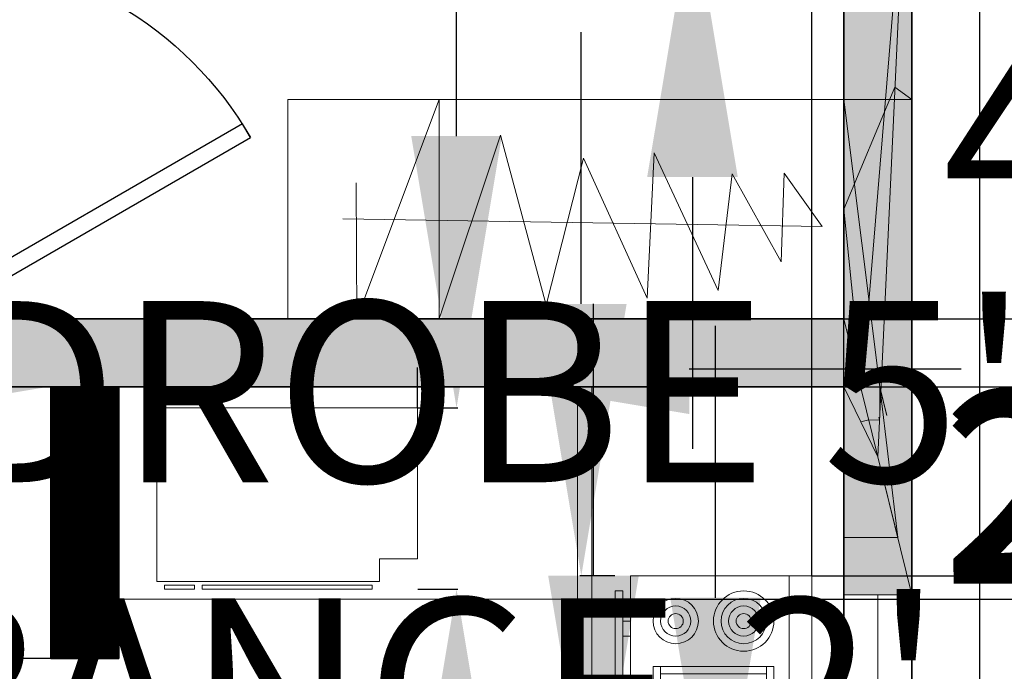
# Model space of a CAD drawing. Units: inches. Extents: x 2838 to 4029, y 1041 to 1915.
# Tile 10 of 16: x 3510 to 3640, y 1460 to 1546. Entities that reach past the tile are written whole.
import ezdxf

# ---------------------------------------------------------------- set-up
doc = ezdxf.new("R2010")
doc.units = ezdxf.units.IN
doc.header["$MEASUREMENT"] = 0
for name, color, linetype, lineweight in [('A-ANNO-DIMS', 2, 'Continuous', 18), ('A-DOOR', 3, 'Continuous', 25), ('A-EQPM', 8, 'Continuous', 18), ('A-FLOR', 7, 'Continuous', 25), ('A-FLOR-CASE', 8, 'Continuous', 18), ('A-GLAZ', 4, 'Continuous', 18), ('A-REFR', 8, 'Continuous', 13), ('A-WALL', 7, 'Continuous', 35), ('A-WALL-PATT', 252, 'Continuous', 13)]:
    doc.layers.add(name, color=color, linetype=linetype, lineweight=lineweight)
doc.styles.get("Standard").update_dxf_attribs({"font": 'arial.ttf'})
doc.dimstyles.get("Standard").update_dxf_attribs({"dimtxt": 24, "dimasz": 36, "dimexe": 0.18, "dimexo": 0.0625, "dimgap": 0.09, "dimtad": 0, "dimtih": 1, "dimtoh": 1, "dimdec": 0, "dimzin": 0, "dimdsep": 46, "dimlunit": 3, "dimtxsty": 'Standard', "dimcen": 0.09, "dimadec": 0, "dimazin": 0, "dimtfac": 1, "dimtdec": 0, "dimtofl": 0, "dimtmove": 0, "dimatfit": 3, "dimfxl": 1, "dimtolj": 1, "dimtzin": 0, "dimarcsym": 0})

# ---------------------------------------------------------------- blocks, each defined once
blk = doc.blocks.new('*U3')
for p, q in [((-40, 0), (-40, 6)), ((0, 0), (0, 6))]:
    blk.add_line(p, q)
blk.add_lwpolyline([(0, 0), (-20, -34.64), (-21.52, -33.77), (-1.52, 0.88)], close=True)
blk.add_arc((0, 0), 40, 180, 240)
blk = doc.blocks.new('Range-Oven - 30 in top')
for p, q in [((0, -3), (30, -3)), ((12, -6), (18, -6)), ((13, -20), (13, -6)), ((14, -6), (14, -20)), ((15, -20), (15, -6)), ((16, -6), (16, -20)), ((17, -20), (17, -6)), ((18, -20), (12, -20)), ((6, -24), (6, -25)), ((8, -25), (8, -24)), ((22, -25), (22, -24)), ((24, -24), (24, -25))]:
    blk.add_line(p, q)
for points in [[(0, -24), (0, 0), (30, 0), (30, -24)], [(12, -21), (12, -5), (18, -5), (18, -21)], [(2, -26), (2, -25), (28, -25), (28, -26)]]:
    blk.add_lwpolyline(points, close=True)
for centre, radius in [((6, -9), 4), ((6, -9), 3), ((24, -9), 3), ((6, -9), 2), ((24, -9), 2), ((6, -9), 1), ((24, -9), 1), ((24, -18), 4), ((6, -18), 3), ((24, -18), 3), ((6, -18), 2), ((24, -18), 2), ((6, -18), 1), ((24, -18), 1)]:
    blk.add_circle(centre, radius)
blk = doc.blocks.new('Base Cabinet 1 Door - side')
for p, q in [((-24, 33.5), (-23.5, 33.5)), ((-24, 29.5), (-24, 33.5)), ((-23.5, 33.5), (-23.5, 29.5)), ((-23.5, 29.5), (-24, 29.5)), ((-24, 6), (-24, 28.5)), ((-24, 28.5), (-23.5, 28.5)), ((-23.5, 28.5), (-23.5, 6)), ((-23.5, 6), (-24, 6)), ((-20, 5), (-23, 5)), ((-20, 0), (-20, 5))]:
    blk.add_line(p, q)
blk.add_lwpolyline([(-23, 5), (-23, 34.5), (0, 34.5), (0, 0), (-20, 0)])
blk = doc.blocks.new('*D17')
at = {"layer": 'A-ANNO-DIMS', "color": 0, "lineweight": -2, "transparency": 16777216}
for p, q in [((3627.79, 1671.3), (3713.18, 1671.3)), ((3713, 1635.3), (3713, 1443.64)), ((3713, 1227.3), (3713, 1418.95)), ((3627.79, 1191.3), (3713.18, 1191.3))]:
    blk.add_line(p, q, dxfattribs=at)
at = {"layer": 'A-ANNO-DIMS', "color": 0, "transparency": 16777216}
for points in [[(3707, 1635.3), (3719, 1635.3), (3713, 1671.3)], [(3707, 1227.3), (3719, 1227.3), (3713, 1191.3)]]:
    blk.add_solid(points, dxfattribs=at)
at = {"layer": 'Defpoints', "color": 0, "transparency": 16777216}
for p in [(3627.73, 1671.3), (3627.73, 1191.3), (3713, 1191.3)]:
    blk.add_point(p, dxfattribs=at)
at = {"layer": 'A-ANNO-DIMS', "color": 0, "transparency": 16777216, "insert": (3713, 1431.3), "char_height": 24, "attachment_point": 5}
blk.add_mtext("\\A1;40'", dxfattribs=at)
blk = doc.blocks.new('WIN-48')
blk.add_line((4.5, 48), (4.5, 0))
blk.add_lwpolyline([(0, 48), (9, 48), (9, 0), (0, 0)], close=True)
blk = doc.blocks.new('WARDROBE-RAIL')
for p, q in [((1.86, 0), (12.76, 29.05)), ((12.76, 29.05), (12.76, 0)), ((12.76, 0), (20.9, 24.31)), ((20.9, 24.31), (26.94, 1.83)), ((26.94, 1.83), (31.9, 21.29)), ((31.9, 21.29), (40.3, 2.75)), ((40.3, 2.75), (41.22, 21.97)), ((41.22, 21.97), (49.7, 3.76)), ((49.7, 3.76), (51.56, 19.2)), ((51.56, 19.2), (58.03, 7.54)), ((58.03, 7.54), (58.45, 19.29)), ((58.45, 19.29), (63.49, 12.24)), ((1.8, 18), (1.86, 0)), ((63.49, 12.24), (0, 13.24)), ((0, 13.24), (63.49, 12.24))]:
    blk.add_line(p, q)
blk = doc.blocks.new('*D27')
at = {"layer": 'A-ANNO-DIMS', "color": 0, "lineweight": -2, "transparency": 16777216}
for p, q in [((3598.68, 1614.31), (3598.68, 1650.31)), ((3598.68, 1650.31), (3634.68, 1650.31)), ((3601.19, 1578.31), (3598.5, 1578.31)), ((3601.19, 1561.16), (3598.5, 1561.16)), ((3598.68, 1525.16), (3598.68, 1489.16))]:
    blk.add_line(p, q, dxfattribs=at)
at = {"layer": 'A-ANNO-DIMS', "color": 0, "transparency": 16777216}
for points in [[(3592.68, 1614.31), (3604.68, 1614.31), (3598.68, 1578.31)], [(3592.68, 1525.16), (3604.68, 1525.16), (3598.68, 1561.16)]]:
    blk.add_solid(points, dxfattribs=at)
at = {"layer": 'Defpoints', "color": 0, "transparency": 16777216}
for p in [(3598.68, 1578.31), (3601.25, 1578.31), (3601.25, 1561.16)]:
    blk.add_point(p, dxfattribs=at)
at = {"layer": 'A-ANNO-DIMS', "color": 0, "transparency": 16777216, "insert": (3820.96, 1650.31), "char_height": 24, "attachment_point": 5}
blk.add_mtext('\\A1;NIGHTSTAND 1\'-5" TYP.', dxfattribs=at)
blk = doc.blocks.new('*D28')
at = {"layer": 'A-ANNO-DIMS', "color": 0, "lineweight": -2, "transparency": 16777216}
for p, q in [((3565.25, 1580.88), (3529.25, 1580.88)), ((3601.25, 1578.37), (3601.25, 1581.06)), ((3617.82, 1578.37), (3617.82, 1581.06)), ((3653.82, 1580.88), (3689.82, 1580.88))]:
    blk.add_line(p, q, dxfattribs=at)
at = {"layer": 'A-ANNO-DIMS', "color": 0, "transparency": 16777216}
for points in [[(3565.25, 1586.88), (3565.25, 1574.88), (3601.25, 1580.88)], [(3653.82, 1586.88), (3653.82, 1574.88), (3617.82, 1580.88)]]:
    blk.add_solid(points, dxfattribs=at)
at = {"layer": 'Defpoints', "color": 0, "transparency": 16777216}
for p in [(3617.82, 1580.88), (3601.25, 1578.31), (3617.82, 1578.31)]:
    blk.add_point(p, dxfattribs=at)
at = {"layer": 'A-ANNO-DIMS', "color": 0, "transparency": 16777216, "insert": (3789.89, 1580.88), "char_height": 24, "attachment_point": 5}
blk.add_mtext('\\A1;1\'-4 1/2" TYP.', dxfattribs=at)
blk = doc.blocks.new('*D33')
at = {"layer": 'A-ANNO-DIMS', "color": 0, "lineweight": -2, "transparency": 16777216}
for p, q in [((3601.73, 1469.45), (3601.73, 1505.45)), ((3603.48, 1433.45), (3601.55, 1433.45)), ((3603.48, 1421.37), (3601.55, 1421.37)), ((3601.73, 1385.37), (3601.73, 1349.37)), ((3601.73, 1349.37), (3565.73, 1349.37))]:
    blk.add_line(p, q, dxfattribs=at)
at = {"layer": 'A-ANNO-DIMS', "color": 0, "transparency": 16777216}
for points in [[(3595.73, 1469.45), (3607.73, 1469.45), (3601.73, 1433.45)], [(3595.73, 1385.37), (3607.73, 1385.37), (3601.73, 1421.37)]]:
    blk.add_solid(points, dxfattribs=at)
at = {"layer": 'Defpoints', "color": 0, "transparency": 16777216}
for p in [(3603.54, 1433.45), (3601.73, 1421.37), (3603.54, 1421.37)]:
    blk.add_point(p, dxfattribs=at)
at = {"layer": 'A-ANNO-DIMS', "color": 0, "transparency": 16777216, "insert": (3496.18, 1349.37), "char_height": 24, "attachment_point": 5}
blk.add_mtext('\\A1;TAP 1\'-0"', dxfattribs=at)
blk = doc.blocks.new('*D41')
at = {"layer": 'A-ANNO-DIMS', "color": 0, "lineweight": -2, "transparency": 16777216}
for p, q in [((3284.24, 1506.2), (3284.24, 1496.56)), ((3347.73, 1506.2), (3347.73, 1496.56)), ((3248.24, 1496.74), (3212.24, 1496.74)), ((3383.73, 1496.74), (3419.73, 1496.74))]:
    blk.add_line(p, q, dxfattribs=at)
at = {"layer": 'A-ANNO-DIMS', "color": 0, "transparency": 16777216}
for points in [[(3248.24, 1502.74), (3248.24, 1490.74), (3284.24, 1496.74)], [(3383.73, 1502.74), (3383.73, 1490.74), (3347.73, 1496.74)]]:
    blk.add_solid(points, dxfattribs=at)
at = {"layer": 'Defpoints', "color": 0, "transparency": 16777216}
for p in [(3284.24, 1506.26), (3347.73, 1506.26), (3347.73, 1496.74)]:
    blk.add_point(p, dxfattribs=at)
at = {"layer": 'A-ANNO-DIMS', "color": 0, "transparency": 16777216, "insert": (3624.81, 1496.74), "char_height": 24, "attachment_point": 5}
blk.add_mtext('\\A1;WARDROBE 5\'-3 1/2" TYP.', dxfattribs=at)
blk = doc.blocks.new('*D47')
at = {"layer": 'A-ANNO-DIMS', "color": 0, "lineweight": -2, "transparency": 16777216}
for p, q in [((3493.47, 1640.5), (3493.47, 1676.5)), ((3493.47, 1676.5), (3529.47, 1676.5)), ((3489.85, 1604.5), (3493.65, 1604.5)), ((3489.85, 1579.95), (3493.65, 1579.95)), ((3493.47, 1543.95), (3493.47, 1507.95))]:
    blk.add_line(p, q, dxfattribs=at)
at = {"layer": 'A-ANNO-DIMS', "color": 0, "transparency": 16777216}
for points in [[(3487.47, 1640.5), (3499.47, 1640.5), (3493.47, 1604.5)], [(3487.47, 1543.95), (3499.47, 1543.95), (3493.47, 1579.95)]]:
    blk.add_solid(points, dxfattribs=at)
at = {"layer": 'Defpoints', "color": 0, "transparency": 16777216}
for p in [(3489.78, 1604.5), (3493.47, 1604.5), (3489.78, 1579.95)]:
    blk.add_point(p, dxfattribs=at)
at = {"layer": 'A-ANNO-DIMS', "color": 0, "transparency": 16777216, "insert": (3643.85, 1676.5), "char_height": 24, "attachment_point": 5}
blk.add_mtext('\\A1;BASIN 2\'-0 1/2"', dxfattribs=at)
blk = doc.blocks.new('*D49')
at = {"layer": 'A-ANNO-DIMS', "color": 0, "lineweight": -2, "transparency": 16777216}
for p, q in [((3336.37, 1426.68), (3336.37, 1412.92)), ((3427.37, 1426.68), (3427.37, 1412.92)), ((3372.37, 1413.1), (3391.37, 1413.1)), ((3427.37, 1413.1), (3463.37, 1413.1))]:
    blk.add_line(p, q, dxfattribs=at)
at = {"layer": 'A-ANNO-DIMS', "color": 0, "transparency": 16777216}
for points in [[(3372.37, 1419.1), (3372.37, 1407.1), (3336.37, 1413.1)], [(3391.37, 1419.1), (3391.37, 1407.1), (3427.37, 1413.1)]]:
    blk.add_solid(points, dxfattribs=at)
at = {"layer": 'Defpoints', "color": 0, "transparency": 16777216}
for p in [(3336.37, 1426.75), (3427.37, 1426.75), (3427.37, 1413.1)]:
    blk.add_point(p, dxfattribs=at)
at = {"layer": 'A-ANNO-DIMS', "color": 0, "transparency": 16777216, "insert": (3595.36, 1413.1), "char_height": 24, "attachment_point": 5}
blk.add_mtext('\\A1;DINING SET 7\'-7"', dxfattribs=at)
blk = doc.blocks.new('*D53')
at = {"layer": 'A-ANNO-DIMS', "color": 0, "lineweight": -2, "transparency": 16777216}
for p, q in [((3583.96, 1508.36), (3583.96, 1544.36)), ((3588.4, 1472.36), (3583.78, 1472.36)), ((3588.4, 1442.36), (3583.78, 1442.36)), ((3583.96, 1406.36), (3583.96, 1370.36))]:
    blk.add_line(p, q, dxfattribs=at)
at = {"layer": 'A-ANNO-DIMS', "color": 0, "transparency": 16777216}
for points in [[(3577.96, 1508.36), (3589.96, 1508.36), (3583.96, 1472.36)], [(3577.96, 1406.36), (3589.96, 1406.36), (3583.96, 1442.36)]]:
    blk.add_solid(points, dxfattribs=at)
at = {"layer": 'Defpoints', "color": 0, "transparency": 16777216}
for p in [(3588.46, 1472.36), (3583.96, 1442.36), (3588.46, 1442.36)]:
    blk.add_point(p, dxfattribs=at)
at = {"layer": 'A-ANNO-DIMS', "color": 0, "transparency": 16777216, "insert": (3583.96, 1457.36), "char_height": 24, "attachment_point": 5}
blk.add_mtext('\\A1;RANGE 2\'-6"', dxfattribs=at)
blk = doc.blocks.new('*D55')
at = {"layer": 'A-ANNO-DIMS', "color": 0, "lineweight": -2, "transparency": 16777216}
for p, q in [((3491.76, 1499.78), (3455.76, 1499.78)), ((3527.76, 1494.67), (3527.76, 1499.96)), ((3562.26, 1494.67), (3562.26, 1499.96)), ((3598.26, 1499.78), (3634.26, 1499.78))]:
    blk.add_line(p, q, dxfattribs=at)
at = {"layer": 'A-ANNO-DIMS', "color": 0, "transparency": 16777216}
for points in [[(3491.76, 1505.78), (3491.76, 1493.78), (3527.76, 1499.78)], [(3598.26, 1505.78), (3598.26, 1493.78), (3562.26, 1499.78)]]:
    blk.add_solid(points, dxfattribs=at)
at = {"layer": 'Defpoints', "color": 0, "transparency": 16777216}
for p in [(3527.76, 1499.78), (3527.76, 1494.6), (3562.26, 1494.6)]:
    blk.add_point(p, dxfattribs=at)
at = {"layer": 'A-ANNO-DIMS', "color": 0, "transparency": 16777216, "insert": (3260.33, 1499.78), "char_height": 24, "attachment_point": 5}
blk.add_mtext('\\A1;BASE CABINET 2\'-10 1/2"', dxfattribs=at)
blk = doc.blocks.new('*D56')
at = {"layer": 'A-ANNO-DIMS', "color": 0, "lineweight": -2, "transparency": 16777216}
for p, q in [((3567.44, 1530.6), (3567.44, 1566.6)), ((3567.44, 1566.6), (3603.44, 1566.6)), ((3562.33, 1494.6), (3567.62, 1494.6)), ((3562.33, 1470.6), (3567.62, 1470.6)), ((3567.44, 1434.6), (3567.44, 1398.6))]:
    blk.add_line(p, q, dxfattribs=at)
at = {"layer": 'A-ANNO-DIMS', "color": 0, "transparency": 16777216}
for points in [[(3561.44, 1530.6), (3573.44, 1530.6), (3567.44, 1494.6)], [(3561.44, 1434.6), (3573.44, 1434.6), (3567.44, 1470.6)]]:
    blk.add_solid(points, dxfattribs=at)
at = {"layer": 'Defpoints', "color": 0, "transparency": 16777216}
for p in [(3562.26, 1494.6), (3567.44, 1494.6), (3562.26, 1470.6)]:
    blk.add_point(p, dxfattribs=at)
at = {"layer": 'A-ANNO-DIMS', "color": 0, "transparency": 16777216, "insert": (3635.63, 1566.6), "char_height": 24, "attachment_point": 5}
blk.add_mtext('\\A1;2\'-0"', dxfattribs=at)
blk = doc.blocks.new('*D57')
at = {"layer": 'A-ANNO-DIMS', "color": 0, "lineweight": -2, "transparency": 16777216}
for p, q in [((3585.57, 1472.38), (3585.57, 1508.38)), ((3590.9, 1436.38), (3585.39, 1436.38)), ((3590.9, 1400.38), (3585.39, 1400.38)), ((3585.57, 1364.38), (3585.57, 1328.38))]:
    blk.add_line(p, q, dxfattribs=at)
at = {"layer": 'A-ANNO-DIMS', "color": 0, "transparency": 16777216}
for points in [[(3579.57, 1472.38), (3591.57, 1472.38), (3585.57, 1436.38)], [(3579.57, 1364.38), (3591.57, 1364.38), (3585.57, 1400.38)]]:
    blk.add_solid(points, dxfattribs=at)
at = {"layer": 'Defpoints', "color": 0, "transparency": 16777216}
for p in [(3590.97, 1436.38), (3585.57, 1400.38), (3590.97, 1400.38)]:
    blk.add_point(p, dxfattribs=at)
at = {"layer": 'A-ANNO-DIMS', "color": 0, "transparency": 16777216, "insert": (3585.57, 1418.38), "char_height": 24, "attachment_point": 5}
blk.add_mtext('\\A1;DOUBLE SINK 3\'-0"', dxfattribs=at)
blk = doc.blocks.new('*D73')
at = {"layer": 'A-ANNO-DIMS', "color": 0, "lineweight": -2, "transparency": 16777216}
for p, q in [((3461.038746, 1200.359846), (3461.038746, 1711.702346)), ((3618.731626, 1200.359846), (3618.731626, 1711.702346)), ((3425.038746, 1711.522346), (3389.038746, 1711.522346)), ((3654.731626, 1711.522346), (3690.731626, 1711.522346))]:
    blk.add_line(p, q, dxfattribs=at)
at = {"layer": 'A-ANNO-DIMS', "color": 0, "transparency": 16777216}
for points in [[(3425.038746, 1717.522346), (3425.038746, 1705.522346), (3461.038746, 1711.522346)], [(3654.731626, 1717.522346), (3654.731626, 1705.522346), (3618.731626, 1711.522346)]]:
    blk.add_solid(points, dxfattribs=at)
at = {"layer": 'Defpoints', "color": 0, "transparency": 16777216}
for p in [(3618.731626, 1711.522346), (3461.038746, 1200.297346), (3618.731626, 1200.297346)]:
    blk.add_point(p, dxfattribs=at)
at = {"layer": 'A-ANNO-DIMS', "color": 0, "transparency": 16777216, "insert": (3539.885186, 1711.522346), "char_height": 24, "attachment_point": 5}
blk.add_mtext('\\A1;13\'-1 1/2"', dxfattribs=at)
blk = doc.blocks.new('*D78')
at = {"layer": 'A-ANNO-DIMS', "color": 0, "lineweight": -2, "transparency": 16777216}
for p, q in [((3667.956626, 1590.394218), (3667.956626, 1626.394218)), ((3498.794126, 1554.394218), (3668.136626, 1554.394218)), ((3498.638013, 1506.394218), (3668.136626, 1506.394218)), ((3667.956626, 1470.394218), (3667.956626, 1434.394218))]:
    blk.add_line(p, q, dxfattribs=at)
at = {"layer": 'A-ANNO-DIMS', "color": 0, "transparency": 16777216}
for points in [[(3661.956626, 1590.394218), (3673.956626, 1590.394218), (3667.956626, 1554.394218)], [(3661.956626, 1470.394218), (3673.956626, 1470.394218), (3667.956626, 1506.394218)]]:
    blk.add_solid(points, dxfattribs=at)
at = {"layer": 'Defpoints', "color": 0, "transparency": 16777216}
for p in [(3498.731626, 1554.394218), (3667.956626, 1554.394218), (3498.575513, 1506.394218)]:
    blk.add_point(p, dxfattribs=at)
at = {"layer": 'A-ANNO-DIMS', "color": 0, "transparency": 16777216, "insert": (3667.956626, 1530.394218), "char_height": 24, "attachment_point": 5}
blk.add_mtext('\\A1;4\'-0"', dxfattribs=at)
blk = doc.blocks.new('*D79')
at = {"layer": 'A-ANNO-DIMS', "color": 0, "lineweight": -2, "transparency": 16777216}
for p, q in [((3379.05, 1400.64), (3379.05, 1711.7)), ((3454.63, 1398.31), (3454.63, 1711.7)), ((3415.05, 1711.52), (3418.63, 1711.52)), ((3454.63, 1711.52), (3490.63, 1711.52))]:
    blk.add_line(p, q, dxfattribs=at)
at = {"layer": 'A-ANNO-DIMS', "color": 0, "transparency": 16777216}
for points in [[(3415.05, 1717.52), (3415.05, 1705.52), (3379.05, 1711.52)], [(3418.63, 1717.52), (3418.63, 1705.52), (3454.63, 1711.52)]]:
    blk.add_solid(points, dxfattribs=at)
at = {"layer": 'Defpoints', "color": 0, "transparency": 16777216}
for p in [(3454.63, 1711.52), (3379.05, 1400.57), (3454.63, 1398.25)]:
    blk.add_point(p, dxfattribs=at)
at = {"layer": 'A-ANNO-DIMS', "color": 0, "transparency": 16777216, "insert": (3550.65, 1711.52), "char_height": 24, "attachment_point": 5}
blk.add_mtext('\\A1;6\'-3 1/2"', dxfattribs=at)
blk = doc.blocks.new('*D82')
at = {"layer": 'A-ANNO-DIMS', "color": 0, "lineweight": -2, "transparency": 16777216}
for p, q in [((3405.73, 1573.06), (3405.73, 1081.89)), ((3441.73, 1569.23), (3441.73, 1081.89)), ((3369.73, 1082.07), (3333.73, 1082.07)), ((3477.73, 1082.07), (3513.73, 1082.07))]:
    blk.add_line(p, q, dxfattribs=at)
at = {"layer": 'A-ANNO-DIMS', "color": 0, "transparency": 16777216}
for points in [[(3369.73, 1088.07), (3369.73, 1076.07), (3405.73, 1082.07)], [(3477.73, 1088.07), (3477.73, 1076.07), (3441.73, 1082.07)]]:
    blk.add_solid(points, dxfattribs=at)
at = {"layer": 'Defpoints', "color": 0, "transparency": 16777216}
for p in [(3405.73, 1573.12), (3441.73, 1569.3), (3441.73, 1082.07)]:
    blk.add_point(p, dxfattribs=at)
at = {"layer": 'A-ANNO-DIMS', "color": 0, "transparency": 16777216, "insert": (3545.71, 1082.07), "char_height": 24, "attachment_point": 5}
blk.add_mtext('\\A1;3\'-0"', dxfattribs=at)
blk = doc.blocks.new('*D87')
at = {"layer": 'A-ANNO-DIMS', "color": 0, "lineweight": -2, "transparency": 16777216}
for p, q in [((3227.506626, 1497.394218), (3227.506626, 1533.394218)), ((3513.669126, 1461.394218), (3227.326626, 1461.394218)), ((3513.669126, 1425.394218), (3227.326626, 1425.394218)), ((3227.506626, 1389.394218), (3227.506626, 1353.394218))]:
    blk.add_line(p, q, dxfattribs=at)
at = {"layer": 'A-ANNO-DIMS', "color": 0, "transparency": 16777216}
for points in [[(3221.506626, 1497.394218), (3233.506626, 1497.394218), (3227.506626, 1461.394218)], [(3221.506626, 1389.394218), (3233.506626, 1389.394218), (3227.506626, 1425.394218)]]:
    blk.add_solid(points, dxfattribs=at)
at = {"layer": 'Defpoints', "color": 0, "transparency": 16777216}
for p in [(3227.506626, 1461.394218), (3513.731626, 1461.394218), (3513.731626, 1425.394218)]:
    blk.add_point(p, dxfattribs=at)
at = {"layer": 'A-ANNO-DIMS', "color": 0, "transparency": 16777216, "insert": (3227.506626, 1443.394218), "char_height": 24, "attachment_point": 5}
blk.add_mtext('\\A1;3\'-0"', dxfattribs=at)
blk = doc.blocks.new('*D89')
at = {"layer": 'A-ANNO-DIMS', "color": 0, "lineweight": -2, "transparency": 16777216}
for p, q in [((3618.79, 1497.39), (3668.14, 1497.39)), ((3667.96, 1461.39), (3667.96, 1450.56)), ((3667.96, 1414.73), (3667.96, 1425.56)), ((3618.79, 1378.73), (3668.14, 1378.73))]:
    blk.add_line(p, q, dxfattribs=at)
at = {"layer": 'A-ANNO-DIMS', "color": 0, "transparency": 16777216}
for points in [[(3661.96, 1461.39), (3673.96, 1461.39), (3667.96, 1497.39)], [(3661.96, 1414.73), (3673.96, 1414.73), (3667.96, 1378.73)]]:
    blk.add_solid(points, dxfattribs=at)
at = {"layer": 'Defpoints', "color": 0, "transparency": 16777216}
for p in [(3618.73, 1497.39), (3667.96, 1497.39), (3618.73, 1378.73)]:
    blk.add_point(p, dxfattribs=at)
at = {"layer": 'A-ANNO-DIMS', "color": 0, "transparency": 16777216, "insert": (3667.96, 1438.06), "char_height": 24, "attachment_point": 5}
blk.add_mtext('\\A1;9\'-10 1/2"', dxfattribs=at)
blk = doc.blocks.new('*D90')
at = {"layer": 'A-ANNO-DIMS', "color": 0, "lineweight": -2, "transparency": 16777216}
for p, q in [((3667.96, 1457.85), (3667.96, 1493.85)), ((3618.79, 1421.85), (3668.14, 1421.85)), ((3618.79, 1378.73), (3668.14, 1378.73)), ((3667.96, 1342.73), (3667.96, 1306.73))]:
    blk.add_line(p, q, dxfattribs=at)
at = {"layer": 'A-ANNO-DIMS', "color": 0, "transparency": 16777216}
for points in [[(3661.96, 1457.85), (3673.96, 1457.85), (3667.96, 1421.85)], [(3661.96, 1342.73), (3673.96, 1342.73), (3667.96, 1378.73)]]:
    blk.add_solid(points, dxfattribs=at)
at = {"layer": 'Defpoints', "color": 0, "transparency": 16777216}
for p in [(3618.73, 1421.85), (3667.96, 1421.85), (3618.73, 1378.73)]:
    blk.add_point(p, dxfattribs=at)
at = {"layer": 'A-ANNO-DIMS', "color": 0, "transparency": 16777216, "insert": (3667.96, 1400.29), "char_height": 24, "attachment_point": 5}
blk.add_mtext('\\A1;3\'-7"', dxfattribs=at)
blk = doc.blocks.new('*D91')
at = {"layer": 'A-ANNO-DIMS', "color": 0, "lineweight": -2, "transparency": 16777216}
for p, q in [((3227.506626, 1533.394218), (3227.506626, 1569.394218)), ((3522.669126, 1497.394218), (3227.326626, 1497.394218)), ((3522.669126, 1461.394218), (3227.326626, 1461.394218)), ((3227.506626, 1425.394218), (3227.506626, 1389.394218))]:
    blk.add_line(p, q, dxfattribs=at)
at = {"layer": 'A-ANNO-DIMS', "color": 0, "transparency": 16777216}
for points in [[(3221.506626, 1533.394218), (3233.506626, 1533.394218), (3227.506626, 1497.394218)], [(3221.506626, 1425.394218), (3233.506626, 1425.394218), (3227.506626, 1461.394218)]]:
    blk.add_solid(points, dxfattribs=at)
at = {"layer": 'Defpoints', "color": 0, "transparency": 16777216}
for p in [(3522.731626, 1497.394218), (3227.506626, 1461.394218), (3522.731626, 1461.394218)]:
    blk.add_point(p, dxfattribs=at)
at = {"layer": 'A-ANNO-DIMS', "color": 0, "transparency": 16777216, "insert": (3227.506626, 1479.394218), "char_height": 24, "attachment_point": 5}
blk.add_mtext('\\A1;3\'-0"', dxfattribs=at)
blk = doc.blocks.new('*D93')
at = {"layer": 'A-ANNO-DIMS', "color": 0, "lineweight": -2, "transparency": 16777216}
for p, q in [((3227.51, 1438.06), (3227.51, 1474.06)), ((3227.51, 1474.06), (3263.51, 1474.06)), ((3522.67, 1402.06), (3227.33, 1402.06)), ((3522.67, 1378.73), (3227.33, 1378.73)), ((3227.51, 1342.73), (3227.51, 1306.73))]:
    blk.add_line(p, q, dxfattribs=at)
at = {"layer": 'A-ANNO-DIMS', "color": 0, "transparency": 16777216}
for points in [[(3221.51, 1438.06), (3233.51, 1438.06), (3227.51, 1402.06)], [(3221.51, 1342.73), (3233.51, 1342.73), (3227.51, 1378.73)]]:
    blk.add_solid(points, dxfattribs=at)
at = {"layer": 'Defpoints', "color": 0, "transparency": 16777216}
for p in [(3227.51, 1402.06), (3522.73, 1402.06), (3522.73, 1378.73)]:
    blk.add_point(p, dxfattribs=at)
at = {"layer": 'A-ANNO-DIMS', "color": 0, "transparency": 16777216, "insert": (3331.65, 1474.06), "char_height": 24, "attachment_point": 5}
blk.add_mtext('\\A1;1\'-11 1/2"', dxfattribs=at)
blk = doc.blocks.new('*D94')
at = {"layer": 'A-ANNO-DIMS', "color": 0, "lineweight": -2, "transparency": 16777216}
for p, q in [((3667.96, 1533.39), (3667.96, 1569.39)), ((3585.44, 1497.39), (3668.14, 1497.39)), ((3585.44, 1469.25), (3668.14, 1469.25)), ((3667.96, 1433.25), (3667.96, 1397.25))]:
    blk.add_line(p, q, dxfattribs=at)
at = {"layer": 'A-ANNO-DIMS', "color": 0, "transparency": 16777216}
for points in [[(3661.96, 1533.39), (3673.96, 1533.39), (3667.96, 1497.39)], [(3661.96, 1433.25), (3673.96, 1433.25), (3667.96, 1469.25)]]:
    blk.add_solid(points, dxfattribs=at)
at = {"layer": 'Defpoints', "color": 0, "transparency": 16777216}
for p in [(3585.37, 1497.39), (3585.37, 1469.25), (3667.96, 1469.25)]:
    blk.add_point(p, dxfattribs=at)
at = {"layer": 'A-ANNO-DIMS', "color": 0, "transparency": 16777216, "insert": (3667.96, 1483.32), "char_height": 24, "attachment_point": 5}
blk.add_mtext('\\A1;2\'-4"', dxfattribs=at)
blk = doc.blocks.new('*D101')
at = {"layer": 'A-ANNO-DIMS', "color": 0, "lineweight": -2, "transparency": 16777216}
for p, q in [((3461.04, 1200.36), (3461.04, 1711.7)), ((3486.18, 1200.36), (3486.18, 1711.7)), ((3425.04, 1711.52), (3389.04, 1711.52)), ((3522.18, 1711.52), (3558.18, 1711.52))]:
    blk.add_line(p, q, dxfattribs=at)
at = {"layer": 'A-ANNO-DIMS', "color": 0, "transparency": 16777216}
for points in [[(3425.04, 1717.52), (3425.04, 1705.52), (3461.04, 1711.52)], [(3522.18, 1717.52), (3522.18, 1705.52), (3486.18, 1711.52)]]:
    blk.add_solid(points, dxfattribs=at)
at = {"layer": 'Defpoints', "color": 0, "transparency": 16777216}
for p in [(3486.18, 1711.52), (3461.04, 1200.3), (3486.18, 1200.3)]:
    blk.add_point(p, dxfattribs=at)
at = {"layer": 'A-ANNO-DIMS', "color": 0, "transparency": 16777216, "insert": (3590.37, 1711.52), "char_height": 24, "attachment_point": 5}
blk.add_mtext('\\A1;2\'-1"', dxfattribs=at)
blk = doc.blocks.new('*D104')
at = {"layer": 'A-ANNO-DIMS', "color": 0, "lineweight": -2, "transparency": 16777216}
for p, q in [((3667.956626, 1533.394218), (3667.956626, 1569.394218)), ((3618.794126, 1497.394218), (3668.136626, 1497.394218)), ((3614.522024, 1472.357294), (3668.136626, 1472.357294)), ((3667.956626, 1436.357294), (3667.956626, 1400.357294))]:
    blk.add_line(p, q, dxfattribs=at)
at = {"layer": 'A-ANNO-DIMS', "color": 0, "transparency": 16777216}
for points in [[(3661.956626, 1533.394218), (3673.956626, 1533.394218), (3667.956626, 1497.394218)], [(3661.956626, 1436.357294), (3673.956626, 1436.357294), (3667.956626, 1472.357294)]]:
    blk.add_solid(points, dxfattribs=at)
at = {"layer": 'Defpoints', "color": 0, "transparency": 16777216}
for p in [(3618.731626, 1497.394218), (3614.459524, 1472.357294), (3667.956626, 1472.357294)]:
    blk.add_point(p, dxfattribs=at)
at = {"layer": 'A-ANNO-DIMS', "color": 0, "transparency": 16777216, "insert": (3667.956626, 1484.875756), "char_height": 24, "attachment_point": 5}
blk.add_mtext('\\A1;2\'-1"', dxfattribs=at)
blk = doc.blocks.new('*D105')
at = {"layer": 'A-ANNO-DIMS', "color": 0, "lineweight": -2, "transparency": 16777216}
for p, q in [((3614.46, 1472.42), (3614.46, 1711.7)), ((3618.73, 1469.91), (3618.73, 1711.7)), ((3578.46, 1711.52), (3542.46, 1711.52)), ((3654.73, 1711.52), (3690.73, 1711.52))]:
    blk.add_line(p, q, dxfattribs=at)
at = {"layer": 'A-ANNO-DIMS', "color": 0, "transparency": 16777216}
for points in [[(3578.46, 1717.52), (3578.46, 1705.52), (3614.46, 1711.52)], [(3654.73, 1717.52), (3654.73, 1705.52), (3618.73, 1711.52)]]:
    blk.add_solid(points, dxfattribs=at)
at = {"layer": 'Defpoints', "color": 0, "transparency": 16777216}
for p in [(3618.73, 1711.52), (3614.46, 1472.36), (3618.73, 1469.85)]:
    blk.add_point(p, dxfattribs=at)
at = {"layer": 'A-ANNO-DIMS', "color": 0, "transparency": 16777216, "insert": (3750.68, 1711.52), "char_height": 24, "attachment_point": 5}
blk.add_mtext('\\A1;0\'-4 1/2"', dxfattribs=at)
blk = doc.blocks.new('*D107')
at = {"layer": 'A-ANNO-DIMS', "color": 0, "lineweight": -2, "transparency": 16777216}
for p, q in [((3667.96, 1436.38), (3667.96, 1472.38)), ((3610.53, 1400.38), (3668.14, 1400.38)), ((3618.79, 1378.73), (3668.14, 1378.73)), ((3667.96, 1342.73), (3667.96, 1306.73)), ((3667.96, 1306.73), (3631.96, 1306.73))]:
    blk.add_line(p, q, dxfattribs=at)
at = {"layer": 'A-ANNO-DIMS', "color": 0, "transparency": 16777216}
for points in [[(3661.96, 1436.38), (3673.96, 1436.38), (3667.96, 1400.38)], [(3661.96, 1342.73), (3673.96, 1342.73), (3667.96, 1378.73)]]:
    blk.add_solid(points, dxfattribs=at)
at = {"layer": 'Defpoints', "color": 0, "transparency": 16777216}
for p in [(3610.47, 1400.38), (3618.73, 1378.73), (3667.96, 1378.73)]:
    blk.add_point(p, dxfattribs=at)
at = {"layer": 'A-ANNO-DIMS', "color": 0, "transparency": 16777216, "insert": (3573.14, 1306.73), "char_height": 24, "attachment_point": 5}
blk.add_mtext('\\A1;1\'-9 1/2"', dxfattribs=at)

msp = doc.modelspace()

# ---------------------------------------------------------------- hatches: boundary and pattern name
at = {"layer": 'A-WALL-PATT'}
h = msp.add_hatch(color=256, dxfattribs=at)
h.dxf.hatch_style = 1
h.paths.add_polyline_path([(3427.52, 1671.3), (3360.91, 1671.3), (3360.91, 1662.3), (3396.73, 1662.3), (3396.73, 1554.39), (3397.12, 1554.39, -0.007312), (3398.53, 1554.41), (3405.73, 1554.41), (3405.73, 1662.3), (3427.52, 1662.3)])
h.paths.add_polyline_path([(3546.42, 1671.3), (3451.52, 1671.3), (3451.52, 1662.3), (3489.73, 1662.3), (3489.73, 1592.86, -0.016107), (3489.73, 1591.9), (3489.73, 1578.3), (3441.73, 1578.3), (3441.73, 1569.3), (3489.73, 1569.3), (3489.73, 1554.41), (3498.73, 1554.41), (3498.73, 1662.3), (3546.42, 1662.3)])
h.paths.add_polyline_path([(3627.73, 1671.3), (3594.42, 1671.3), (3594.42, 1662.3), (3618.73, 1662.3), (3618.73, 1634.03), (3627.73, 1634.03)])
h.paths.add_polyline_path([(3627.73, 1586.03), (3618.73, 1586.03), (3618.73, 1506.39), (3545.12, 1506.39), (3489.73, 1506.39), (3489.73, 1497.39), (3513.73, 1497.39), (3618.73, 1497.39), (3618.73, 1469.85), (3627.73, 1469.85)])
h.paths.add_polyline_path([(3627.73, 1421.85), (3618.73, 1421.85), (3618.73, 1378.73), (3522.73, 1378.73), (3513.73, 1378.73), (3461.04, 1378.73), (3461.04, 1369.73), (3513.73, 1369.73), (3618.73, 1369.73), (3618.73, 1320.94), (3627.73, 1320.94)])
h.paths.add_polyline_path([(3627.73, 1272.94), (3618.73, 1272.94), (3618.73, 1200.3), (3599.07, 1200.3), (3599.07, 1191.3), (3627.73, 1191.3)])
h.paths.add_polyline_path([(3551.07, 1200.3), (3510.18, 1200.3), (3510.18, 1191.3), (3551.07, 1191.3)])
h.paths.add_polyline_path([(3486.18, 1200.3), (3461.04, 1200.3), (3461.04, 1398.25), (3454.63, 1398.25), (3454.63, 1200.3), (3432.45, 1200.3), (3432.45, 1191.3), (3486.18, 1191.3)])
h.paths.add_polyline_path([(3300.73, 1200.3), (3276.73, 1200.3), (3276.73, 1391.57), (3331.05, 1391.57), (3331.05, 1400.57), (3276.73, 1400.57), (3276.73, 1432.17), (3267.73, 1432.17), (3267.73, 1191.3), (3300.73, 1191.3)])
h = msp.add_hatch(dxfattribs=at)
h.set_pattern_fill('ANSI31', color=256)
h.paths.add_polyline_path([(3522.73, 1497.39), (3513.73, 1497.39), (3513.73, 1461.39), (3522.73, 1461.39)])
h.paths.add_polyline_path([(3522.73, 1425.39), (3513.73, 1425.39), (3513.73, 1378.73), (3522.73, 1378.73), (3522.73, 1402.06)])

# ---------------------------------------------------------------- linework, layer by layer
at = {"layer": 'A-FLOR'}
msp.add_lwpolyline([(3527.95, 1182.3), (3636.73, 1182.3), (3636.73, 1680.3), (3258.73, 1680.3), (3258.73, 1182.3), (3267.73, 1182.3)], dxfattribs=at)
at = {"layer": 'A-FLOR-CASE'}
msp.add_line((3583.47, 1497.39), (3583.47, 1469.25), dxfattribs=at)
msp.add_lwpolyline([(3545.12, 1535.45), (3618.73, 1535.45), (3618.73, 1506.39), (3545.12, 1506.39)], close=True, dxfattribs=at)
for points in [[(3585.37, 1469.25), (3522.73, 1469.25), (3522.73, 1497.39), (3618.73, 1497.39), (3618.73, 1469.25)], [(3585.37, 1378.73), (3618.73, 1378.73), (3618.73, 1497.39), (3585.37, 1497.39), (3585.37, 1402.06)]]:
    msp.add_lwpolyline(points, dxfattribs=at)
at = {"layer": 'A-REFR'}
for p, q in [((3627.73, 1586.03), (3623.23, 1488.12)), ((3627.73, 1469.85), (3627.73, 1586.03)), ((3621.1, 1497.39), (3626.92, 1568.43)), ((3625.48, 1537.08), (3618.73, 1520.92)), ((3627.73, 1535.45), (3625.48, 1537.08)), ((3623.47, 1497.39), (3618.73, 1535.45)), ((3618.73, 1535.45), (3627.73, 1535.45)), ((3618.73, 1520.92), (3621.1, 1497.39)), ((3618.73, 1506.39), (3627.73, 1469.85)), ((3623.23, 1488.12), (3618.73, 1497.39)), ((3618.73, 1497.39), (3620.98, 1492.76)), ((3623.47, 1497.39), (3618.73, 1497.39)), ((3618.73, 1497.39), (3623.23, 1488.12)), ((3623.47, 1493.34), (3623.47, 1497.39)), ((3623.47, 1497.39), (3624.41, 1493.6)), ((3623.94, 1495.5), (3623.47, 1497.39)), ((3623.47, 1497.39), (3623.66, 1497.39)), ((3623.66, 1497.39), (3623.47, 1497.39)), ((3623.47, 1497.39), (3623.47, 1497.39)), ((3625.87, 1477.41), (3623.47, 1497.39)), ((3623.66, 1497.39), (3623.66, 1497.39)), ((3624.41, 1493.6), (3623.94, 1495.5)), ((3623.94, 1495.5), (3623.94, 1495.5)), ((3620.98, 1492.76), (3622.03, 1493.01)), ((3622.03, 1493.01), (3623.45, 1492.95)), ((3623.45, 1492.95), (3623.36, 1493.34)), ((3623.36, 1493.34), (3623.47, 1493.34)), ((3624.41, 1493.6), (3624.41, 1493.6)), ((3624.41, 1493.6), (3624.41, 1493.6)), ((3623.23, 1488.12), (3625.87, 1477.41)), ((3625.87, 1477.41), (3618.73, 1477.41)), ((3618.73, 1477.41), (3625.87, 1477.41))]:
    msp.add_line(p, q, dxfattribs=at)
at = {"layer": 'A-WALL'}
for p, q in [((3627.73, 1191.3), (3627.73, 1671.3)), ((3618.73, 1506.39), (3618.73, 1662.3)), ((3618.73, 1586.03), (3618.73, 1506.39)), ((3627.73, 1421.85), (3627.73, 1586.03)), ((3618.73, 1506.39), (3489.73, 1506.39)), ((3618.73, 1506.39), (3489.73, 1506.39)), ((3491.37, 1506.39), (3618.73, 1506.39)), ((3618.73, 1497.39), (3489.73, 1497.39)), ((3489.73, 1497.39), (3513.73, 1497.39)), ((3513.73, 1461.39), (3513.73, 1497.39)), ((3513.73, 1497.39), (3513.73, 1461.39)), ((3522.73, 1461.39), (3522.73, 1497.39)), ((3522.73, 1461.39), (3522.73, 1497.39)), ((3522.73, 1497.39), (3618.73, 1497.39)), ((3618.73, 1378.73), (3618.73, 1497.39)), ((3618.73, 1497.39), (3618.73, 1469.85)), ((3618.73, 1469.85), (3618.73, 1421.85)), ((3618.73, 1421.85), (3618.73, 1469.25)), ((3618.73, 1469.25), (3618.73, 1421.85)), ((3522.73, 1461.39), (3513.73, 1461.39)), ((3513.73, 1461.39), (3522.73, 1461.39))]:
    msp.add_line(p, q, dxfattribs=at)
msp.add_lwpolyline([(3372.73, 1191.3), (3627.73, 1191.3), (3627.73, 1671.3), (3267.73, 1671.3), (3267.73, 1191.3), (3300.73, 1191.3)], dxfattribs=at)

# ---------------------------------------------------------------- block references
at = {"layer": 'A-DOOR', "xscale": -1.200513446172712, "yscale": 1.200513446172712, "zscale": 1.200513446172712, "rotation": 90}
msp.add_blockref('*U3', (3498.58, 1506.39), dxfattribs=at)
at = {"layer": 'A-EQPM', "rotation": 270}
msp.add_blockref('Range-Oven - 30 in top', (3614.46, 1472.36), dxfattribs=at)
at = {"layer": 'A-FLOR-CASE'}
msp.add_blockref('WARDROBE-RAIL', (3552.37, 1506.39), dxfattribs=at)
at = {"layer": 'A-FLOR-CASE', "rotation": 90}
msp.add_blockref('Base Cabinet 1 Door - side', (3562.26, 1494.6), dxfattribs=at)
at = {"layer": 'A-GLAZ'}
msp.add_blockref('WIN-48', (3618.73, 1421.85), dxfattribs=at)

# ---------------------------------------------------------------- dimensions: what is measured, and where the dimension line sits
at = {"layer": 'A-ANNO-DIMS'}
for base, p1, p2, picture, middle in [((3454.63, 1711.52), (3379.05, 1400.57), (3454.63, 1398.25), '*D79', (3550.65, 1711.52)), ((3618.73, 1711.52), (3461.04, 1200.3), (3618.73, 1200.3), '*D73', (3539.89, 1711.52)), ((3618.73, 1711.52), (3614.46, 1472.36), (3618.73, 1469.85), '*D105', (3750.68, 1711.52)), ((3486.18, 1711.52), (3461.04, 1200.3), (3486.18, 1200.3), '*D101', (3590.37, 1711.52)), ((3441.73, 1082.07), (3405.73, 1573.12), (3441.73, 1569.3), '*D82', (3545.71, 1082.07))]:
    dim = msp.add_linear_dim(base=base, p1=p1, p2=p2, dimstyle='Standard', override={"dimdec": 1, "dimlfac": 1, "dimrnd": 0, "dimzin": 1, "dimdsep": 46, "dimlunit": 4, "dimfrac": 2}, dxfattribs=at)
    dim.commit()
    dim.dimension.update_dxf_attribs({"geometry": picture, "text_midpoint": middle})
for base, p1, p2, angle, text, picture, middle in [((3493.4667, 1604.5013), (3489.7841, 1579.9504), (3489.7841, 1604.5013), 90, 'BASIN <>', '*D47', (3643.8514, 1676.5013)), ((3598.6826, 1578.3092), (3601.2549, 1561.1604), (3601.2549, 1578.3092), 90, 'NIGHTSTAND <> TYP.', '*D27', (3820.9609, 1650.3092)), ((3527.76, 1499.78), (3562.26, 1494.6), (3527.76, 1494.6), 180, 'BASE CABINET <>', '*D55', (3260.33, 1499.78)), ((3583.96, 1442.36), (3588.46, 1472.36), (3588.46, 1442.36), 270, 'RANGE <>', '*D53', (3583.96, 1457.36)), ((3585.57, 1400.38), (3590.97, 1436.38), (3590.97, 1400.38), 270, 'DOUBLE SINK <>', '*D57', (3585.57, 1418.38)), ((3601.73, 1421.37), (3603.54, 1433.45), (3603.54, 1421.37), 270, 'TAP <>', '*D33', (3496.18, 1349.37))]:
    dim = msp.add_linear_dim(base=base, p1=p1, p2=p2, angle=angle, text=text, dimstyle='Standard', override={"dimdec": 1, "dimlfac": 1, "dimrnd": 0, "dimzin": 1, "dimdsep": 46, "dimlunit": 4, "dimfrac": 2}, dxfattribs=at)
    dim.commit()
    dim.dimension.update_dxf_attribs({"geometry": picture, "text_midpoint": middle})
for base, p1, p2, override, picture, middle in [((3713, 1191.3), (3627.73, 1671.3), (3627.73, 1191.3), {"dimclrd": 0, "dimclre": 0, "dimclrt": 0}, '*D17', (3713, 1431.3)), ((3667.96, 1554.39), (3498.58, 1506.39), (3498.73, 1554.39), {"dimdec": 1, "dimlfac": 1, "dimrnd": 0, "dimzin": 1, "dimdsep": 46, "dimlunit": 4, "dimfrac": 2}, '*D78', (3667.96, 1530.39)), ((3567.44, 1494.6), (3562.26, 1470.6), (3562.26, 1494.6), {"dimdec": 1, "dimlfac": 1, "dimrnd": 0, "dimzin": 1, "dimdsep": 46, "dimlunit": 4, "dimfrac": 2}, '*D56', (3635.63, 1566.6)), ((3227.51, 1461.39), (3522.73, 1497.39), (3522.73, 1461.39), {"dimdec": 1, "dimlfac": 1, "dimrnd": 0, "dimzin": 1, "dimdsep": 46, "dimlunit": 4, "dimfrac": 2}, '*D91', (3227.51, 1479.39)), ((3667.96, 1469.25), (3585.37, 1497.39), (3585.37, 1469.25), {"dimdec": 1, "dimlfac": 1, "dimrnd": 0, "dimzin": 1, "dimdsep": 46, "dimlunit": 4, "dimfrac": 2}, '*D94', (3667.96, 1483.32)), ((3667.96, 1472.36), (3618.73, 1497.39), (3614.46, 1472.36), {"dimdec": 1, "dimlfac": 1, "dimrnd": 0, "dimzin": 1, "dimdsep": 46, "dimlunit": 4, "dimfrac": 2}, '*D104', (3667.96, 1484.88)), ((3227.51, 1461.39), (3513.73, 1425.39), (3513.73, 1461.39), {"dimdec": 1, "dimlfac": 1, "dimrnd": 0, "dimzin": 1, "dimdsep": 46, "dimlunit": 4, "dimfrac": 2}, '*D87', (3227.51, 1443.39)), ((3227.51, 1402.06), (3522.73, 1378.73), (3522.73, 1402.06), {"dimdec": 1, "dimlfac": 1, "dimrnd": 0, "dimzin": 1, "dimdsep": 46, "dimlunit": 4, "dimfrac": 2}, '*D93', (3331.65, 1474.06)), ((3667.96, 1497.39), (3618.73, 1378.73), (3618.73, 1497.39), {"dimdec": 1, "dimlfac": 1, "dimrnd": 0, "dimzin": 1, "dimdsep": 46, "dimlunit": 4, "dimfrac": 2}, '*D89', (3667.96, 1438.06)), ((3667.96, 1421.85), (3618.73, 1378.73), (3618.73, 1421.85), {"dimdec": 1, "dimlfac": 1, "dimrnd": 0, "dimzin": 1, "dimdsep": 46, "dimlunit": 4, "dimfrac": 2}, '*D90', (3667.96, 1400.29)), ((3667.9566, 1378.7272), (3610.4672, 1400.3841), (3618.7316, 1378.7272), {"dimdec": 1, "dimlfac": 1, "dimrnd": 0, "dimzin": 1, "dimdsep": 46, "dimlunit": 4, "dimfrac": 2}, '*D107', (3573.1354, 1306.7272))]:
    dim = msp.add_linear_dim(base=base, p1=p1, p2=p2, angle=90, dimstyle='Standard', override=override, dxfattribs=at)
    dim.commit()
    dim.dimension.update_dxf_attribs({"geometry": picture, "text_midpoint": middle})
for base, p1, p2, text, picture, middle in [((3617.82, 1580.88), (3601.25, 1578.31), (3617.82, 1578.31), '<> TYP.', '*D28', (3789.89, 1580.88)), ((3347.73, 1496.74), (3284.24, 1506.26), (3347.73, 1506.26), 'WARDROBE <> TYP.', '*D41', (3624.81, 1496.74)), ((3427.37, 1413.1), (3336.37, 1426.75), (3427.37, 1426.75), 'DINING SET <>', '*D49', (3595.36, 1413.1))]:
    dim = msp.add_linear_dim(base=base, p1=p1, p2=p2, text=text, dimstyle='Standard', override={"dimdec": 1, "dimlfac": 1, "dimrnd": 0, "dimzin": 1, "dimdsep": 46, "dimlunit": 4, "dimfrac": 2}, dxfattribs=at)
    dim.commit()
    dim.dimension.update_dxf_attribs({"geometry": picture, "text_midpoint": middle})

doc.saveas('drawing.dxf')
